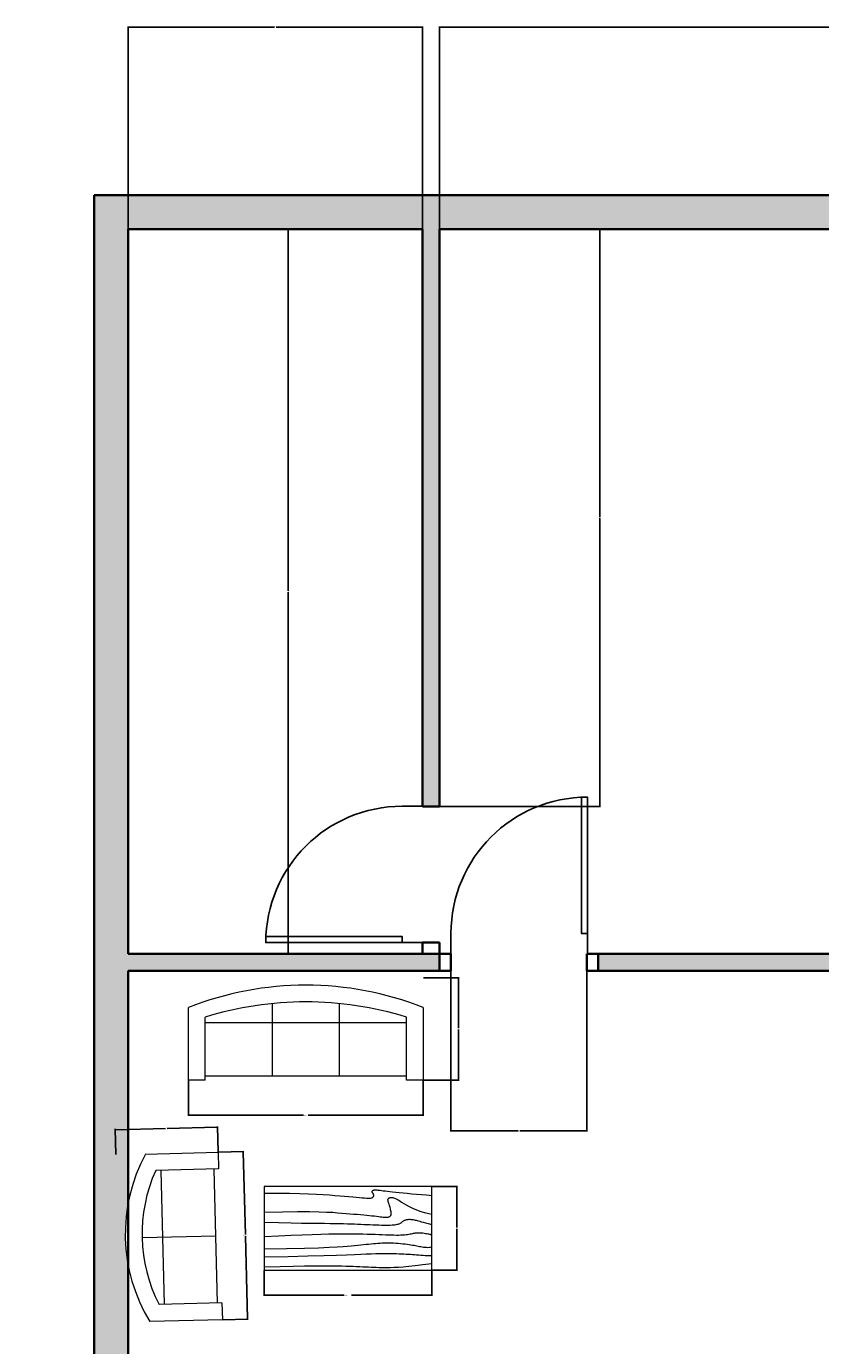
# Model space of a CAD drawing. Units: inches. Extents: x 1563 to 2428, y 777 to 1464.
# Tile 10 of 11: x 2007 to 2218, y 1115 to 1464. Entities that reach past the tile are written whole.
import ezdxf

# ---------------------------------------------------------------- set-up
doc = ezdxf.new("R2010")
doc.units = ezdxf.units.IN
for name, color, linetype, lineweight in [('A-ANNO-DIMS', 2, 'Continuous', 18), ('A-DOOR', 4, 'Continuous', 25), ('A-FURN', 9, 'Continuous', 18), ('A-WALL', 7, 'Continuous', 35), ('A-WALL-PATT', 8, 'Continuous', 13)]:
    doc.layers.add(name, color=color, linetype=linetype, lineweight=lineweight)
doc.styles.get("Standard").update_dxf_attribs({"font": 'arial.ttf'})
doc.dimstyles.get("Standard").update_dxf_attribs({"dimtxt": 0.18, "dimasz": 0.18, "dimexe": 0.18, "dimexo": 0.0625, "dimgap": 0.09, "dimtad": 0, "dimtih": 1, "dimtoh": 1, "dimdec": 4, "dimzin": 0, "dimdsep": 46, "dimtxsty": 'Standard', "dimcen": 0.09, "dimadec": 0, "dimazin": 0, "dimtfac": 1, "dimtdec": 4, "dimtofl": 0, "dimtmove": 0, "dimatfit": 3, "dimfxl": 1, "dimtolj": 1, "dimtzin": 0, "dimarcsym": 0})

# ---------------------------------------------------------------- blocks, each defined once
blk = doc.blocks.new('*U3')
for p, q in [((0, 0), (0, -6)), ((-40, 0), (-40, -6))]:
    blk.add_line(p, q)
blk.add_lwpolyline([(0, 0), (0, 40), (-1.75, 40), (-1.75, 0)], close=True)
blk.add_arc((0, 0), 40, 90, 180)
blk = doc.blocks.new('*U4')
for p, q in [((0, 0), (0, -6)), ((40, 0), (40, -6))]:
    blk.add_line(p, q)
blk.add_lwpolyline([(0, 0), (0, 40), (1.75, 40), (1.75, 0)], close=True)
blk.add_arc((0, 0), 40, 0, 90)
blk = doc.blocks.new('Sofa - Roundback 7 ft.')
for p, q in [((-12.00002, -32.4421), (-12.00003, -6.5971)), ((11.99997, -32.4421), (11.99998, -6.5971)), ((-36.000027, -34), (-36.000027, -11.4696)), ((-35.999844, -13.3819), (35.9998, -13.3819)), ((35.99998, -34), (35.99998, -11.4696)), ((-36.000027, -32.4421), (35.99998, -32.4421))]:
    blk.add_line(p, q)
for points in [[(-36.000027, -34), (-42.000027, -34), (-42.000027, -8)], [(41.99998, -8), (41.99998, -34), (35.99998, -34)]]:
    blk.add_lwpolyline(points)
for centre, radius, start, end in [((0, -114.25), 114.25, 68.43141, 111.5686), ((-0.00001, -127.1968), 121.1968, 72.72033, 107.2797)]:
    blk.add_arc(centre, radius, start, end)
blk = doc.blocks.new('Sofa - Roundback Loveseat 5 ft.')
for p, q in [((0, -32.44198), (0, -5.99998)), ((-24, -33.99998), (-24, -11.46958)), ((-23.9998, -13.38178), (23.99986, -13.38178)), ((24.00004, -33.99998), (24.00004, -11.46958)), ((-24, -32.44198), (24.00004, -32.44198))]:
    blk.add_line(p, q)
for points in [[(-24, -33.99998), (-30, -33.99998), (-30, -7.99998)], [(30.00004, -7.99998), (30.00004, -33.99998), (24.00004, -33.99998)]]:
    blk.add_lwpolyline(points)
for centre, radius, start, end in [((0, -60.24998), 60.24998, 60.13715, 119.8628), ((0, -61.38438), 55.38444, 64.32083, 115.6792)]:
    blk.add_arc(centre, radius, start, end)
blk = doc.blocks.new('Table - Rectangular Woodgrain 60 x 30 in.')
for p, q in [((0, 0), (0, -30)), ((60, 0), (0, 0)), ((60, -30), (60, 0)), ((0, -30), (60, -30))]:
    blk.add_line(p, q)
for points in [[(0, -2.4), (4.8155, -2.418), (9.0302, -2.4688), (12.709, -2.5477), (15.9167, -2.65), (18.7181, -2.7711), (21.1781, -2.9063), (23.3616, -3.0508), (25.3333, -3.2), (27.1477, -3.3495), (28.8172, -3.4958), (30.3437, -3.636), (31.7291, -3.7667), (32.9756, -3.8849), (34.0849, -3.9875), (35.059, -4.0714), (35.9, -4.1334), (36.6114, -4.1711), (37.2041, -4.1854), (37.6906, -4.1779), (38.0833, -4.15), (38.3948, -4.1034), (38.6375, -4.0396), (38.8239, -3.9602), (38.9666, -3.8667), (39.0764, -3.7608), (39.1573, -3.6448), (39.2116, -3.521), (39.2416, -3.3917), (39.2498, -3.2593), (39.2385, -3.1261), (39.21, -2.9944), (39.1666, -2.8667), (39.111, -2.7447), (39.0468, -2.6281), (38.978, -2.5163), (38.9083, -2.4083), (38.8418, -2.3035), (38.7823, -2.201), (38.7337, -2.1001), (38.7, -2), (38.6844, -1.9003), (38.6875, -1.8021), (38.7094, -1.707), (38.75, -1.6167), (38.8094, -1.5326), (38.8875, -1.4563), (38.9844, -1.3893), (39.1, -1.3333), (39.2351, -1.2896), (39.3937, -1.2583), (39.5804, -1.2396), (39.8, -1.2333), (40.057, -1.2396), (40.3562, -1.2583), (40.7023, -1.2896), (41.1, -1.3333), (41.5547, -1.3895), (42.0755, -1.4573), (42.6721, -1.5361), (43.3542, -1.625), (44.1316, -1.7233), (45.014, -1.8302), (46.0114, -1.9449), (47.1333, -2.0667), (48.3862, -2.1947), (49.7625, -2.3281), (51.2513, -2.4663), (52.8416, -2.6083), (54.5226, -2.7535), (56.2833, -2.9011), (58.1127, -3.0501), (60, -3.2)], [(0, -9.2), (6.5759, -9.0858), (11.9385, -9.0365), (16.2527, -9.0418), (19.6833, -9.0917), (22.3952, -9.1759), (24.5531, -9.2844), (26.322, -9.4069), (27.8666, -9.5333), (29.3241, -9.6553), (30.7203, -9.7719), (32.0532, -9.8837), (33.3208, -9.9917), (34.5213, -10.0965), (35.6526, -10.199), (36.7128, -10.2999), (37.7, -10.4), (38.6129, -10.4996), (39.4531, -10.5969), (40.223, -10.6895), (40.925, -10.775), (41.5613, -10.8512), (42.1344, -10.9156), (42.6465, -10.966), (43.1, -11), (43.4976, -11.0158), (43.8437, -11.0136), (44.143, -10.9942), (44.4, -10.9583), (44.6195, -10.9069), (44.8062, -10.8406), (44.9648, -10.7603), (45.1, -10.6667), (45.2155, -10.5598), (45.3114, -10.4365), (45.3871, -10.2929), (45.4416, -10.125), (45.4743, -9.929), (45.4844, -9.7011), (45.4709, -9.4371), (45.4333, -9.1333), (45.3716, -8.7883), (45.2896, -8.4104), (45.1919, -8.0107), (45.0833, -7.6), (44.9685, -7.1893), (44.8521, -6.7896), (44.7388, -6.4117), (44.6333, -6.0667), (44.54, -5.7628), (44.4614, -5.4979), (44.4001, -5.2675), (44.3583, -5.0667), (44.3384, -4.8909), (44.3427, -4.7354), (44.3736, -4.5956), (44.4333, -4.4667), (44.5236, -4.3453), (44.6427, -4.2333), (44.7884, -4.1339), (44.9583, -4.05), (45.1501, -3.9849), (45.3614, -3.9417), (45.59, -3.9234), (45.8333, -3.9333), (46.0915, -3.9749), (46.3734, -4.0531), (46.6906, -4.1736), (47.0542, -4.3417), (47.4756, -4.5629), (47.9661, -4.8427), (48.5372, -5.1866), (49.2, -5.6), (49.9676, -6.0844), (50.8594, -6.625), (51.8965, -7.2031), (53.1, -7.8), (54.491, -8.3969), (56.0906, -8.975), (57.9199, -9.5156), (60, -10)], [(0, -12.8), (5.1847, -12.9322), (9.6213, -13.0323), (13.3963, -13.1059), (16.5958, -13.1583), (19.3063, -13.1952), (21.614, -13.2219), (23.6054, -13.2439), (25.3666, -13.2667), (26.9728, -13.2947), (28.4531, -13.3281), (29.8256, -13.3663), (31.1083, -13.4083), (32.3191, -13.4535), (33.476, -13.501), (34.597, -13.5501), (35.7, -13.6), (36.7984, -13.6497), (37.8875, -13.6979), (38.9578, -13.743), (40, -13.7833), (41.0047, -13.8174), (41.9625, -13.8438), (42.864, -13.8607), (43.7, -13.8667), (44.4631, -13.8604), (45.1552, -13.8417), (45.7801, -13.8104), (46.3416, -13.7667), (46.8439, -13.7104), (47.2906, -13.6417), (47.6858, -13.5604), (48.0333, -13.4667), (48.3375, -13.3608), (48.6042, -13.2448), (48.8396, -13.121), (49.05, -12.9917), (49.2417, -12.8593), (49.4208, -12.7261), (49.5937, -12.5944), (49.7667, -12.4667), (49.9452, -12.3451), (50.1323, -12.2313), (50.3303, -12.1268), (50.5416, -12.0333), (50.7686, -11.9524), (51.0135, -11.8854), (51.2788, -11.8341), (51.5666, -11.8), (51.8785, -11.7843), (52.2116, -11.7865), (52.562, -11.8059), (52.926, -11.8417), (53.2998, -11.8931), (53.6795, -11.9594), (54.0614, -12.0397), (54.4416, -12.1333), (54.8223, -12.2401), (55.2293, -12.3625), (55.6942, -12.5037), (56.2489, -12.6667), (56.9251, -12.8547), (57.7545, -13.0708), (58.7689, -13.3182), (60, -13.6)], [(0, -18), (5.124, -17.7273), (9.6609, -17.5057), (13.6705, -17.3303), (17.2125, -17.1958), (20.3467, -17.0973), (23.1328, -17.0297), (25.6307, -16.9878), (27.9, -16.9667), (29.9928, -16.9617), (31.9302, -16.9703), (33.7254, -16.9907), (35.3917, -17.0208), (36.9423, -17.0588), (38.3906, -17.1026), (39.7499, -17.1503), (41.0333, -17.2), (42.2519, -17.2496), (43.4073, -17.2969), (44.4986, -17.3395), (45.525, -17.375), (46.4858, -17.4012), (47.3802, -17.4156), (48.2074, -17.416), (48.9667, -17.4), (49.6583, -17.3662), (50.2872, -17.3167), (50.8595, -17.2547), (51.3812, -17.1833), (51.8584, -17.1057), (52.2971, -17.025), (52.7034, -16.9443), (53.0833, -16.8667), (53.443, -16.7951), (53.789, -16.7313), (54.128, -16.6768), (54.4666, -16.6334), (54.8115, -16.6024), (55.1693, -16.5854), (55.5465, -16.5841), (55.95, -16.6), (56.3828, -16.6337), (56.8346, -16.6823), (57.2915, -16.7418), (57.7396, -16.8084), (58.165, -16.878), (58.5539, -16.9469), (58.8924, -17.0111), (59.1666, -17.0667), (59.3679, -17.1107), (59.5078, -17.1438), (59.6032, -17.1675), (59.6708, -17.1833), (59.7275, -17.193), (59.7901, -17.1979), (59.8753, -17.1998), (60, -17.2)], [(0, -22.4), (8.0098, -22.2501), (14.4094, -22.1011), (19.4168, -21.9535), (23.25, -21.8083), (26.1269, -21.6663), (28.2656, -21.5281), (29.884, -21.3947), (31.2, -21.2667), (32.3967, -21.1448), (33.5172, -21.0292), (34.5697, -20.9198), (35.5625, -20.8167), (36.5037, -20.7198), (37.4015, -20.6292), (38.2642, -20.5448), (39.1, -20.4667), (39.9164, -20.3951), (40.7187, -20.3313), (41.5117, -20.2768), (42.3, -20.2333), (43.0883, -20.2024), (43.8812, -20.1854), (44.6836, -20.1841), (45.5, -20.2), (46.3328, -20.234), (47.1747, -20.2844), (48.0163, -20.3488), (48.8479, -20.425), (49.66, -20.5106), (50.4429, -20.6031), (51.1872, -20.7004), (51.8833, -20.8), (52.5246, -20.8999), (53.1166, -20.9995), (53.6681, -21.0983), (54.1875, -21.1958), (54.6834, -21.2919), (55.1646, -21.3859), (55.6394, -21.4777), (56.1167, -21.5667), (56.6028, -21.6515), (57.0961, -21.7266), (57.5929, -21.7852), (58.0896, -21.8208), (58.5823, -21.8268), (59.0674, -21.7964), (59.5412, -21.723), (60, -21.6)], [(0, -25.2), (8.6355, -25.0504), (15.7026, -24.9031), (21.4049, -24.7606), (25.9458, -24.625), (29.529, -24.4988), (32.3578, -24.3844), (34.6359, -24.284), (36.5667, -24.2), (38.3213, -24.1341), (39.9417, -24.0854), (41.437, -24.0523), (42.8167, -24.0333), (44.0901, -24.0268), (45.2667, -24.0313), (46.3557, -24.0451), (47.3667, -24.0667), (48.309, -24.0947), (49.1928, -24.1287), (50.0284, -24.168), (50.826, -24.2125), (51.5959, -24.2617), (52.3483, -24.3151), (53.0935, -24.3725), (53.8417, -24.4334), (54.6009, -24.497), (55.3699, -24.561), (56.1454, -24.6226), (56.9239, -24.6792), (57.7021, -24.7279), (58.4764, -24.7662), (59.2435, -24.7911), (60, -24.8)], [(0, -28.8), (5.6867, -28.6681), (10.45, -28.5698), (14.407, -28.5012), (17.675, -28.4584), (20.3711, -28.4374), (22.6125, -28.4344), (24.5164, -28.4455), (26.2, -28.4667), (27.762, -28.4947), (29.2276, -28.5281), (30.6033, -28.5663), (31.8958, -28.6084), (33.1118, -28.6535), (34.2578, -28.7011), (35.3405, -28.7501), (36.3666, -28.8), (37.3443, -28.8497), (38.288, -28.8974), (39.2137, -28.9412), (40.1375, -28.9792), (41.0753, -29.0093), (42.0432, -29.0297), (43.0572, -29.0384), (44.1333, -29.0333), (45.2936, -29.0114), (46.5843, -28.9641), (48.0579, -28.8816), (49.7666, -28.7542), (51.7629, -28.5721), (54.0989, -28.3255), (56.8272, -28.0048), (60, -27.6)]]:
    blk.add_lwpolyline(points)
blk = doc.blocks.new('*D26')
at = {"layer": 'A-ANNO-DIMS', "color": 0, "lineweight": -2, "transparency": 16777216}
for p, q in [((2050.29, 1184.83), (2050.29, 1175.4)), ((2112.41, 1184.83), (2112.41, 1175.4)), ((2050.47, 1175.58), (2080.75, 1175.58)), ((2112.23, 1175.58), (2081.94, 1175.58))]:
    blk.add_line(p, q, dxfattribs=at)
at = {"layer": 'A-ANNO-DIMS', "color": 0, "transparency": 16777216}
for points in [[(2050.47, 1175.61), (2050.47, 1175.55), (2050.29, 1175.58)], [(2112.23, 1175.61), (2112.23, 1175.55), (2112.41, 1175.58)]]:
    blk.add_solid(points, dxfattribs=at)
at = {"layer": 'Defpoints', "color": 0, "transparency": 16777216}
for p in [(2050.29, 1184.9), (2112.41, 1184.9), (2112.41, 1175.58)]:
    blk.add_point(p, dxfattribs=at)
at = {"layer": 'A-ANNO-DIMS', "color": 0, "transparency": 16777216, "insert": (2081.35, 1175.58), "char_height": 0.18, "attachment_point": 5}
blk.add_mtext('\\A1;SOFA 62', dxfattribs=at)
blk = doc.blocks.new('*D27')
at = {"layer": 'A-ANNO-DIMS', "color": 0, "lineweight": -2, "transparency": 16777216}
for p, q in [((2112.47, 1212.01), (2121.9, 1212.01)), ((2121.72, 1211.83), (2121.72, 1198.63)), ((2121.72, 1185.08), (2121.72, 1198.27)), ((2112.47, 1184.9), (2121.9, 1184.9))]:
    blk.add_line(p, q, dxfattribs=at)
at = {"layer": 'A-ANNO-DIMS', "color": 0, "transparency": 16777216}
for points in [[(2121.69, 1211.83), (2121.75, 1211.83), (2121.72, 1212.01)], [(2121.69, 1185.08), (2121.75, 1185.08), (2121.72, 1184.9)]]:
    blk.add_solid(points, dxfattribs=at)
at = {"layer": 'Defpoints', "color": 0, "transparency": 16777216}
for p in [(2112.41, 1212.01), (2121.72, 1212.01), (2112.41, 1184.9)]:
    blk.add_point(p, dxfattribs=at)
at = {"layer": 'A-ANNO-DIMS', "color": 0, "transparency": 16777216, "insert": (2121.72, 1198.45), "char_height": 0.18, "attachment_point": 5}
blk.add_mtext('\\A1;27', dxfattribs=at)
blk = doc.blocks.new('*D30')
at = {"layer": 'A-ANNO-DIMS', "color": 0, "lineweight": -2, "transparency": 16777216}
for p, q in [((2058.19, 1165.78), (2064.97, 1165.95)), ((2064.79, 1165.77), (2065.33, 1143.95)), ((2065.89, 1121.77), (2065.34, 1143.59)), ((2059.3, 1121.43), (2066.07, 1121.6))]:
    blk.add_line(p, q, dxfattribs=at)
at = {"layer": 'A-ANNO-DIMS', "color": 0, "transparency": 16777216}
for points in [[(2064.82, 1165.77), (2064.76, 1165.77), (2064.79, 1165.95)], [(2065.92, 1121.77), (2065.86, 1121.77), (2065.89, 1121.59)]]:
    blk.add_solid(points, dxfattribs=at)
at = {"layer": 'Defpoints', "color": 0, "transparency": 16777216}
for p in [(2058.13, 1165.78), (2064.79, 1165.95), (2059.24, 1121.43)]:
    blk.add_point(p, dxfattribs=at)
at = {"layer": 'A-ANNO-DIMS', "color": 0, "transparency": 16777216, "insert": (2065.34, 1143.77), "char_height": 0.18, "attachment_point": 5}
blk.add_mtext('\\A1;LOVESEAT 44', dxfattribs=at)
blk = doc.blocks.new('*D31')
at = {"layer": 'A-ANNO-DIMS', "color": 0, "lineweight": -2, "transparency": 16777216}
for p, q in [((2031.03, 1165.17), (2030.86, 1171.94)), ((2031.04, 1171.76), (2044.19, 1172.09)), ((2057.79, 1172.43), (2044.63, 1172.1)), ((2058.13, 1165.84), (2057.96, 1172.61))]:
    blk.add_line(p, q, dxfattribs=at)
at = {"layer": 'A-ANNO-DIMS', "color": 0, "transparency": 16777216}
for points in [[(2031.04, 1171.79), (2031.04, 1171.73), (2030.86, 1171.76)], [(2057.79, 1172.46), (2057.79, 1172.4), (2057.97, 1172.43)]]:
    blk.add_solid(points, dxfattribs=at)
at = {"layer": 'Defpoints', "color": 0, "transparency": 16777216}
for p in [(2030.86, 1171.76), (2031.03, 1165.1), (2058.13, 1165.78)]:
    blk.add_point(p, dxfattribs=at)
at = {"layer": 'A-ANNO-DIMS', "color": 0, "transparency": 16777216, "insert": (2044.41, 1172.09), "char_height": 0.18, "attachment_point": 5}
blk.add_mtext('\\A1;27', dxfattribs=at)
blk = doc.blocks.new('*D34')
at = {"layer": 'A-ANNO-DIMS', "color": 0, "lineweight": -2, "transparency": 16777216}
for p, q in [((2070.3, 1134.48), (2070.3, 1127.71)), ((2114.67, 1134.48), (2114.67, 1127.71)), ((2070.48, 1127.89), (2091.52, 1127.89)), ((2114.49, 1127.89), (2093.45, 1127.89))]:
    blk.add_line(p, q, dxfattribs=at)
at = {"layer": 'A-ANNO-DIMS', "color": 0, "transparency": 16777216}
for points in [[(2070.48, 1127.92), (2070.48, 1127.86), (2070.3, 1127.89)], [(2114.49, 1127.92), (2114.49, 1127.86), (2114.67, 1127.89)]]:
    blk.add_solid(points, dxfattribs=at)
at = {"layer": 'Defpoints', "color": 0, "transparency": 16777216}
for p in [(2070.3, 1134.54), (2114.67, 1134.54), (2114.67, 1127.89)]:
    blk.add_point(p, dxfattribs=at)
at = {"layer": 'A-ANNO-DIMS', "color": 0, "transparency": 16777216, "insert": (2092.49, 1127.89), "char_height": 0.18, "attachment_point": 5}
blk.add_mtext('\\A1;LOW TABLE 44', dxfattribs=at)
blk = doc.blocks.new('*D35')
at = {"layer": 'A-ANNO-DIMS', "color": 0, "lineweight": -2, "transparency": 16777216}
for p, q in [((2114.73, 1156.73), (2121.5, 1156.73)), ((2121.32, 1156.55), (2121.32, 1145.82)), ((2121.32, 1134.72), (2121.32, 1145.46)), ((2114.73, 1134.54), (2121.5, 1134.54))]:
    blk.add_line(p, q, dxfattribs=at)
at = {"layer": 'A-ANNO-DIMS', "color": 0, "transparency": 16777216}
for points in [[(2121.29, 1156.55), (2121.35, 1156.55), (2121.32, 1156.73)], [(2121.29, 1134.72), (2121.35, 1134.72), (2121.32, 1134.54)]]:
    blk.add_solid(points, dxfattribs=at)
at = {"layer": 'Defpoints', "color": 0, "transparency": 16777216}
for p in [(2114.67, 1156.73), (2121.32, 1156.73), (2114.67, 1134.54)]:
    blk.add_point(p, dxfattribs=at)
at = {"layer": 'A-ANNO-DIMS', "color": 0, "transparency": 16777216, "insert": (2121.32, 1145.64), "char_height": 0.18, "attachment_point": 5}
blk.add_mtext('\\A1;22', dxfattribs=at)
blk = doc.blocks.new('*D75')
at = {"layer": 'A-ANNO-DIMS', "color": 0, "lineweight": -2, "transparency": 16777216}
for p, q in [((2034.27, 1410.39), (2034.27, 1464.01)), ((2034.45, 1463.83), (2073.05, 1463.83)), ((2112.09, 1463.83), (2073.49, 1463.83)), ((2112.27, 1410.39), (2112.27, 1464.01))]:
    blk.add_line(p, q, dxfattribs=at)
at = {"layer": 'A-ANNO-DIMS', "color": 0, "transparency": 16777216}
for points in [[(2034.45, 1463.86), (2034.45, 1463.8), (2034.27, 1463.83)], [(2112.09, 1463.86), (2112.09, 1463.8), (2112.27, 1463.83)]]:
    blk.add_solid(points, dxfattribs=at)
at = {"layer": 'Defpoints', "color": 0, "transparency": 16777216}
for p in [(2112.27, 1463.83), (2034.27, 1410.32), (2112.27, 1410.32)]:
    blk.add_point(p, dxfattribs=at)
at = {"layer": 'A-ANNO-DIMS', "color": 0, "transparency": 16777216, "insert": (2073.27, 1463.83), "char_height": 0.18, "attachment_point": 5}
blk.add_mtext('\\A1;78', dxfattribs=at)
blk = doc.blocks.new('*D76')
at = {"layer": 'A-ANNO-DIMS', "color": 0, "lineweight": -2, "transparency": 16777216}
for p, q in [((2116.77, 1410.39), (2116.77, 1464.01)), ((2116.95, 1463.83), (2246.12, 1463.83)), ((2376.09, 1463.83), (2246.92, 1463.83)), ((2376.27, 1410.39), (2376.27, 1464.01))]:
    blk.add_line(p, q, dxfattribs=at)
at = {"layer": 'A-ANNO-DIMS', "color": 0, "transparency": 16777216}
for points in [[(2116.95, 1463.86), (2116.95, 1463.8), (2116.77, 1463.83)], [(2376.09, 1463.86), (2376.09, 1463.8), (2376.27, 1463.83)]]:
    blk.add_solid(points, dxfattribs=at)
at = {"layer": 'Defpoints', "color": 0, "transparency": 16777216}
for p in [(2376.27, 1463.83), (2116.77, 1410.32), (2376.27, 1410.32)]:
    blk.add_point(p, dxfattribs=at)
at = {"layer": 'A-ANNO-DIMS', "color": 0, "transparency": 16777216, "insert": (2246.52, 1463.83), "char_height": 0.18, "attachment_point": 5}
blk.add_mtext('\\A1;259.5', dxfattribs=at)
blk = doc.blocks.new('*D77')
at = {"layer": 'A-ANNO-DIMS', "color": 0, "lineweight": -2, "transparency": 16777216}
for p, q in [((2034.33, 1410.32), (2076.85, 1410.32)), ((2076.67, 1410.14), (2076.67, 1314.51)), ((2076.67, 1218.5), (2076.67, 1314.14)), ((2034.33, 1218.32), (2076.85, 1218.32))]:
    blk.add_line(p, q, dxfattribs=at)
at = {"layer": 'A-ANNO-DIMS', "color": 0, "transparency": 16777216}
for points in [[(2076.64, 1410.14), (2076.7, 1410.14), (2076.67, 1410.32)], [(2076.64, 1218.5), (2076.7, 1218.5), (2076.67, 1218.32)]]:
    blk.add_solid(points, dxfattribs=at)
at = {"layer": 'Defpoints', "color": 0, "transparency": 16777216}
for p in [(2034.27, 1410.32), (2034.27, 1218.32), (2076.67, 1218.32)]:
    blk.add_point(p, dxfattribs=at)
at = {"layer": 'A-ANNO-DIMS', "color": 0, "transparency": 16777216, "insert": (2076.67, 1314.32), "char_height": 0.18, "attachment_point": 5}
blk.add_mtext('\\A1;192', dxfattribs=at)
blk = doc.blocks.new('*D86')
at = {"layer": 'A-ANNO-DIMS', "color": 0, "lineweight": -2, "transparency": 16777216}
for p, q in [((2119.77, 1213.76), (2119.77, 1171.24)), ((2155.77, 1213.76), (2155.77, 1171.24)), ((2119.95, 1171.42), (2137.55, 1171.42)), ((2155.59, 1171.42), (2137.99, 1171.42))]:
    blk.add_line(p, q, dxfattribs=at)
at = {"layer": 'A-ANNO-DIMS', "color": 0, "transparency": 16777216}
for points in [[(2119.95, 1171.45), (2119.95, 1171.39), (2119.77, 1171.42)], [(2155.59, 1171.45), (2155.59, 1171.39), (2155.77, 1171.42)]]:
    blk.add_solid(points, dxfattribs=at)
at = {"layer": 'Defpoints', "color": 0, "transparency": 16777216}
for p in [(2119.77, 1213.82), (2155.77, 1213.82), (2119.77, 1171.42)]:
    blk.add_point(p, dxfattribs=at)
at = {"layer": 'A-ANNO-DIMS', "color": 0, "transparency": 16777216, "insert": (2137.77, 1171.42), "char_height": 0.18, "attachment_point": 5}
blk.add_mtext('\\A1;36', dxfattribs=at)
blk = doc.blocks.new('*D87')
at = {"layer": 'A-ANNO-DIMS', "color": 0, "lineweight": -2, "transparency": 16777216}
for p, q in [((2116.83, 1410.32), (2159.35, 1410.32)), ((2159.17, 1410.14), (2159.17, 1334.01)), ((2159.17, 1257.5), (2159.17, 1333.64)), ((2116.83, 1257.32), (2159.35, 1257.32))]:
    blk.add_line(p, q, dxfattribs=at)
at = {"layer": 'A-ANNO-DIMS', "color": 0, "transparency": 16777216}
for points in [[(2159.14, 1410.14), (2159.2, 1410.14), (2159.17, 1410.32)], [(2159.14, 1257.5), (2159.2, 1257.5), (2159.17, 1257.32)]]:
    blk.add_solid(points, dxfattribs=at)
at = {"layer": 'Defpoints', "color": 0, "transparency": 16777216}
for p in [(2116.77, 1410.32), (2116.77, 1257.32), (2159.17, 1257.32)]:
    blk.add_point(p, dxfattribs=at)
at = {"layer": 'A-ANNO-DIMS', "color": 0, "transparency": 16777216, "insert": (2159.17, 1333.82), "char_height": 0.18, "attachment_point": 5}
blk.add_mtext('\\A1;153', dxfattribs=at)

msp = doc.modelspace()

# ---------------------------------------------------------------- hatches: boundary and pattern name
at = {"layer": 'A-WALL-PATT'}
h = msp.add_hatch(color=256, dxfattribs=at)
h.dxf.hatch_style = 1
h.paths.add_polyline_path([(2385.27, 1419.324), (2025.27, 1419.324), (2025.27, 819.324), (2385.27, 819.324)])
h.paths.add_polyline_path([(2034.27, 1410.324), (2112.27, 1410.324), (2112.27, 1257.324), (2116.77, 1257.324), (2116.77, 1410.324), (2376.27, 1410.324), (2376.27, 1218.324), (2158.77, 1218.324), (2158.77, 1213.824), (2376.27, 1213.824), (2376.27, 1117.824), (2280.27, 1117.824), (2280.27, 1174.824), (2275.77, 1174.824), (2275.77, 1113.324), (2376.27, 1113.324), (2376.27, 828.324), (2214.27, 828.324), (2214.27, 1039.824), (2211.27, 1039.824), (2211.27, 828.324), (2034.27, 828.324), (2034.27, 1039.824), (2172.27, 1039.824), (2172.27, 1044.324), (2034.27, 1044.324), (2034.27, 1136.044, -0.0910221), (2034.27, 1152.131), (2034.27, 1213.824), (2116.77, 1213.824), (2116.77, 1218.324), (2034.27, 1218.324)], flags=16)
h.paths.add_polyline_path([(2106.854, 1222.904), (2106.854, 1221.324), (2070.749, 1221.324), (2070.749, 1222.904)], flags=0)
h.paths.add_polyline_path([(2112.405, 1204.123), (2112.405, 1184.897), (2107.968, 1184.897), (2107.968, 1186.049), (2054.728, 1186.049), (2054.728, 1184.897), (2050.292, 1184.897), (2050.292, 1204.123, -0.1904762)], flags=0)
h.paths.add_polyline_path([(2090.222, 1205.162), (2090.222, 1200.143), (2072.475, 1200.143), (2072.475, 1205.162, -0.0496282)], flags=0)
h.paths.add_polyline_path([(2154.296, 1259.846), (2155.876, 1259.846), (2155.876, 1223.74), (2154.296, 1223.74)], flags=0)
h.paths.add_polyline_path([(2057.091, 1161.316), (2057.976, 1125.833), (2042.473, 1125.447, -0.2279232), (2041.588, 1160.929)], flags=0)
h.paths.add_polyline_path([(2070.302, 1156.728), (2114.669, 1156.728), (2114.669, 1134.544), (2070.302, 1134.544)], flags=0)
h.paths.add_polyline_path([(2098.463, 1153.659), (2098.693, 1153.693), (2098.873, 1153.74), (2099.01, 1153.799), (2099.116, 1153.868), (2099.197, 1153.947), (2099.257, 1154.032), (2099.297, 1154.124), (2099.319, 1154.22), (2099.325, 1154.317), (2099.317, 1154.416), (2099.296, 1154.513), (2099.264, 1154.608), (2099.223, 1154.698), (2099.175, 1154.784), (2099.152, 1154.822), (2099.024, 1155.024), (2098.98, 1155.1), (2098.886, 1155.294), (2098.952, 1155.577), (2099.204, 1155.752), (2099.49, 1155.809), (2099.811, 1155.818), (2100.249, 1155.79), (2100.399, 1155.774), (2100.143, 1155.797), (2099.922, 1155.811), (2099.732, 1155.816), (2099.57, 1155.811), (2099.432, 1155.797), (2099.315, 1155.774), (2099.215, 1155.742), (2099.129, 1155.7), (2099.057, 1155.651), (2099, 1155.594), (2098.956, 1155.532), (2098.926, 1155.465), (2098.91, 1155.395), (2098.907, 1155.322), (2098.919, 1155.249), (2098.944, 1155.175), (2098.98, 1155.1), (2099.024, 1155.024), (2099.073, 1154.947), (2099.124, 1154.867), (2099.239, 1154.68), (2099.35, 1154.353), (2099.273, 1154.02), (2099.025, 1153.78), (2098.599, 1153.668)], flags=0)
h.paths.add_polyline_path([(2102.466, 1148.582), (2102.722, 1148.584), (2102.944, 1148.598), (2103.134, 1148.624), (2103.296, 1148.662), (2103.434, 1148.711), (2103.551, 1148.771), (2103.651, 1148.84), (2103.737, 1148.919), (2103.808, 1149.01), (2103.864, 1149.116), (2103.904, 1149.241), (2103.928, 1149.386), (2103.936, 1149.554), (2103.926, 1149.749), (2103.898, 1149.974), (2103.852, 1150.229), (2103.791, 1150.508), (2103.719, 1150.804), (2103.639, 1151.108), (2103.554, 1151.411), (2103.468, 1151.707), (2103.384, 1151.986), (2103.306, 1152.242), (2103.192, 1152.613), (2103.109, 1152.925), (2103.073, 1153.241), (2103.204, 1153.522), (2103.537, 1153.75), (2103.928, 1153.83), (2104.287, 1153.815), (2104.697, 1153.701), (2104.827, 1153.641), (2104.593, 1153.73), (2104.384, 1153.788), (2104.194, 1153.819), (2104.014, 1153.826), (2103.845, 1153.813), (2103.688, 1153.781), (2103.546, 1153.733), (2103.421, 1153.671), (2103.313, 1153.597), (2103.225, 1153.514), (2103.158, 1153.425), (2103.114, 1153.329), (2103.091, 1153.226), (2103.088, 1153.111), (2103.103, 1152.981), (2103.134, 1152.832), (2103.179, 1152.662), (2103.237, 1152.466), (2103.306, 1152.242), (2103.384, 1151.986), (2103.468, 1151.707), (2103.554, 1151.411), (2103.639, 1151.108), (2103.719, 1150.804), (2103.831, 1150.346), (2103.921, 1149.846), (2103.94, 1149.459), (2103.881, 1149.105), (2103.667, 1148.829), (2103.373, 1148.68), (2103.05, 1148.605), (2102.609, 1148.576)], flags=0)
h.paths.add_polyline_path([(2105.563, 1146.7), (2105.82, 1146.77), (2106.045, 1146.848), (2106.242, 1146.934), (2106.417, 1147.025), (2106.572, 1147.121), (2106.714, 1147.219), (2106.846, 1147.317), (2107.065, 1147.484), (2107.307, 1147.648), (2107.597, 1147.802), (2107.932, 1147.921), (2108.322, 1147.996), (2108.777, 1148.019), (2109.297, 1147.991), (2109.852, 1147.914), (2110.415, 1147.796), (2110.559, 1147.756), (2110.278, 1147.825), (2109.995, 1147.884), (2109.715, 1147.933), (2109.438, 1147.971), (2109.169, 1147.998), (2108.91, 1148.012), (2108.664, 1148.014), (2108.433, 1148.002), (2108.22, 1147.977), (2108.024, 1147.939), (2107.843, 1147.889), (2107.675, 1147.83), (2107.519, 1147.76), (2107.372, 1147.683), (2107.234, 1147.599), (2107.102, 1147.509), (2106.974, 1147.415), (2106.747, 1147.242), (2106.488, 1147.063), (2106.146, 1146.883), (2105.705, 1146.729)], flags=0)
h.paths.add_polyline_path([(2114.376, 1144.033), (2114.426, 1144.021), (2114.436, 1144.02), (2114.305, 1144.051)], flags=0)
h.paths.add_polyline_path([(2242.564, 1401.056), (2376.27, 1401.056), (2376.27, 1300.776), (2242.564, 1300.776)], flags=0)
h.paths.add_polyline_path([(2326.799, 1326.18), (2352.203, 1326.18), (2352.203, 1387.685), (2374.265, 1387.685), (2374.265, 1352.922), (2352.203, 1352.922), (2352.203, 1348.91), (2374.265, 1348.91), (2374.265, 1314.147), (2348.86, 1314.147), (2348.86, 1322.838), (2326.799, 1300.776)], flags=0)
h.paths.add_polyline_path([(2313.978, 1083.124), (2342.025, 1083.124), (2370.073, 1083.124), (2370.073, 977.167), (2342.025, 977.167), (2313.978, 977.167)], flags=0)
h.paths.add_polyline_path([(1834.605, 1034.428), (1914.224, 1034.428), (1914.224, 1038.928), (1614.105, 1038.928), (1614.105, 1034.428), (1830.105, 1034.428), (1830.105, 830.428), (1834.605, 830.428)])

# ---------------------------------------------------------------- linework, layer by layer
at = {"layer": 'A-WALL'}
for p, q in [((2034.27, 1410.324), (2112.27, 1410.324)), ((2034.27, 1218.324), (2034.27, 1410.324)), ((2112.27, 1410.324), (2112.27, 1257.324)), ((2116.77, 1410.324), (2116.77, 1257.324)), ((2116.77, 1410.324), (2376.27, 1410.324)), ((2112.27, 1257.324), (2116.77, 1257.324)), ((2112.27, 1221.324), (2116.77, 1221.324)), ((2112.27, 1221.324), (2112.27, 1218.324)), ((2116.77, 1221.324), (2116.77, 1213.824)), ((2034.27, 1218.324), (2119.77, 1218.324)), ((2119.77, 1218.324), (2119.77, 1213.824)), ((2155.77, 1218.324), (2155.77, 1213.824)), ((2155.77, 1218.324), (2376.27, 1218.324)), ((2158.77, 1218.324), (2158.77, 1213.824)), ((2034.27, 1213.824), (2119.77, 1213.824)), ((2034.27, 1044.324), (2034.27, 1213.824)), ((2155.77, 1213.824), (2376.27, 1213.824))]:
    msp.add_line(p, q, dxfattribs=at)
msp.add_lwpolyline([(2025.27, 1419.324), (2385.27, 1419.324), (2385.27, 819.324), (2025.27, 819.324)], close=True, dxfattribs=at)

# ---------------------------------------------------------------- block references
at = {"layer": 'A-DOOR', "xscale": 0.9026413098436022, "yscale": 0.9026413098436022, "zscale": 0.9026413098436022}
msp.add_blockref('*U3', (2155.876, 1223.74), dxfattribs=at)
at = {"layer": 'A-DOOR', "xscale": 0.9026413098436022, "yscale": 0.9026413098436022, "zscale": 0.9026413098436022, "rotation": 90}
msp.add_blockref('*U4', (2106.854, 1221.324), dxfattribs=at)
at = {"layer": 'A-FURN', "xscale": 0.7394452624391967, "yscale": 0.7394452624391967, "zscale": 0.7394452624391967}
for name, p in [('Sofa - Roundback 7 ft.', (2081.348, 1210.039)), ('Table - Rectangular Woodgrain 60 x 30 in.', (2070.302, 1156.728))]:
    msp.add_blockref(name, p, dxfattribs=at)
at = {"layer": 'A-FURN', "xscale": 0.7394452624391967, "yscale": 0.7394452624391967, "zscale": 0.7394452624391967, "rotation": 91.42884202491504}
msp.add_blockref('Sofa - Roundback Loveseat 5 ft.', (2033.552, 1142.976), dxfattribs=at)

# ---------------------------------------------------------------- dimensions: what is measured, and where the dimension line sits
at = {"layer": 'A-ANNO-DIMS'}
for base, p1, p2, override, picture, middle in [((2112.27, 1463.828), (2034.27, 1410.324), (2112.27, 1410.324), {"dimdec": 0, "dimlfac": 1, "dimrnd": 0, "dimzin": 0, "dimdsep": 46, "dimlunit": 2}, '*D75', (2073.27, 1463.828)), ((2376.27, 1463.828), (2116.77, 1410.324), (2376.27, 1410.324), {"dimdec": 1, "dimlfac": 1, "dimrnd": 0, "dimzin": 0, "dimdsep": 46, "dimlunit": 2}, '*D76', (2246.52, 1463.828))]:
    dim = msp.add_linear_dim(base=base, p1=p1, p2=p2, dimstyle='Standard', override=override, dxfattribs=at)
    dim.commit()
    dim.dimension.update_dxf_attribs({"geometry": picture, "text_midpoint": middle})
for base, p1, p2, angle, picture, middle in [((2076.67, 1218.324), (2034.27, 1410.324), (2034.27, 1218.324), 270, '*D77', (2076.67, 1314.324)), ((2159.17, 1257.324), (2116.77, 1410.324), (2116.77, 1257.324), 270, '*D87', (2159.17, 1333.824)), ((2119.77, 1171.424), (2155.77, 1213.824), (2119.77, 1213.824), 180, '*D86', (2137.77, 1171.424)), ((2121.722, 1212.01), (2112.405, 1184.897), (2112.405, 1212.01), 90, '*D27', (2121.722, 1198.454)), ((2030.862, 1171.757), (2058.132, 1165.78), (2031.028, 1165.104), 181.42884, '*D31', (2044.414, 1172.095)), ((2121.324, 1156.728), (2114.669, 1134.544), (2114.669, 1156.728), 90, '*D35', (2121.324, 1145.636))]:
    dim = msp.add_linear_dim(base=base, p1=p1, p2=p2, angle=angle, dimstyle='Standard', override={"dimdec": 0, "dimlfac": 1, "dimrnd": 0, "dimzin": 0, "dimdsep": 46, "dimlunit": 2}, dxfattribs=at)
    dim.commit()
    dim.dimension.update_dxf_attribs({"geometry": picture, "text_midpoint": middle})
for base, p1, p2, text, picture, middle in [((2112.405, 1175.58), (2050.292, 1184.897), (2112.405, 1184.897), 'SOFA <>', '*D26', (2081.348, 1175.58)), ((2114.669, 1127.889), (2070.302, 1134.544), (2114.669, 1134.544), 'LOW TABLE <>', '*D34', (2092.486, 1127.889))]:
    dim = msp.add_linear_dim(base=base, p1=p1, p2=p2, text=text, dimstyle='Standard', override={"dimdec": 0, "dimlfac": 1, "dimrnd": 0, "dimzin": 0, "dimdsep": 46, "dimlunit": 2}, dxfattribs=at)
    dim.commit()
    dim.dimension.update_dxf_attribs({"geometry": picture, "text_midpoint": middle})
dim = msp.add_linear_dim(base=(2064.785, 1165.946), p1=(2059.238, 1121.427), p2=(2058.132, 1165.78), angle=91.42884, text='LOVESEAT <>', dimstyle='Standard', override={"dimdec": 0, "dimlfac": 1, "dimrnd": 0, "dimzin": 0, "dimdsep": 46, "dimlunit": 2}, dxfattribs=at)
dim.commit()
dim.dimension.update_dxf_attribs({"geometry": '*D30', "text_midpoint": (2065.338, 1143.769)})

doc.saveas('drawing.dxf')
